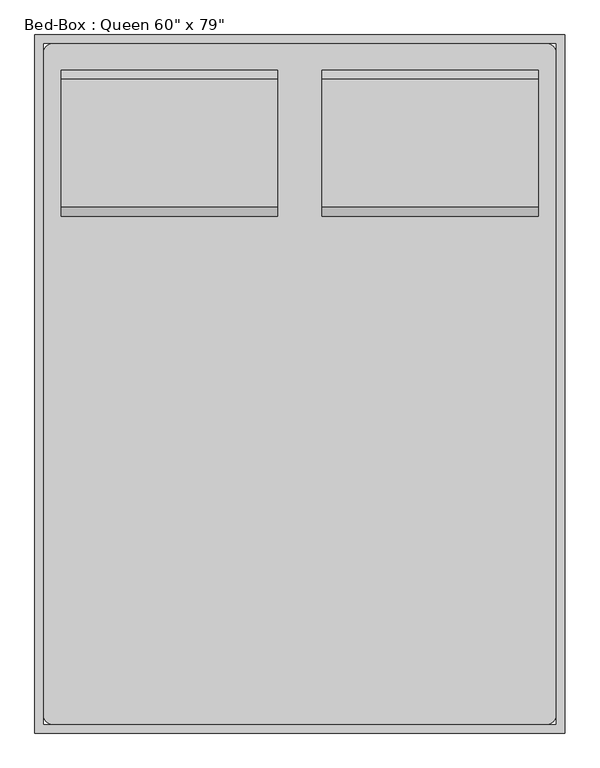
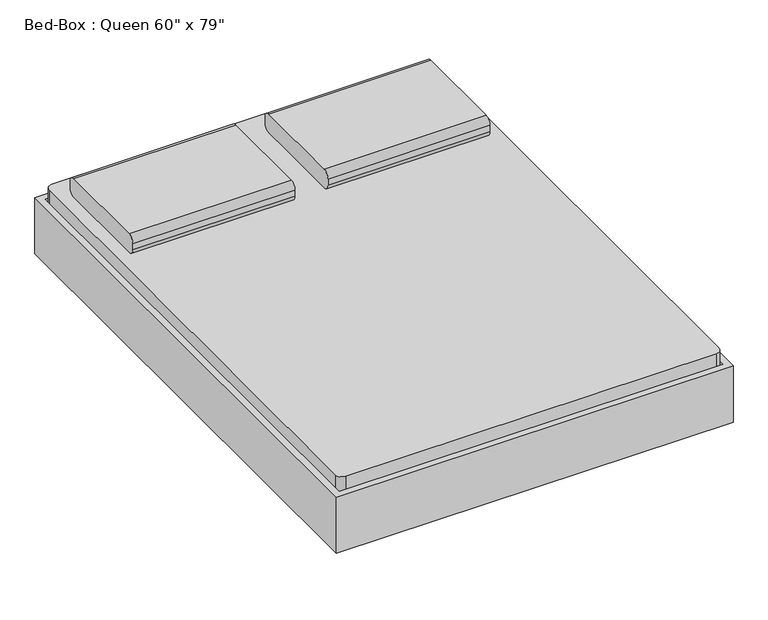
"""IFC4 building model written with IfcOpenShell, lengths in millimetres: furniture geometry."""

from ifc_helpers import new_model, si_unit, point, frame, frame_2d, origin, place, context, project, spatial, polyline, circle_curve, trimmed, segment, composite_curve, outline, extrude, source, transform, mapped, element, save
from ifc_brep_helpers import plane_surface, cylinder_surface, revolved_surface, advanced_brep


def furniture_1d2926bd(model_context):
    return source(origin(), model_context, "Body", "SolidModel", [
        extrude(outline(composite_curve([segment(polyline([(641.8704918, 406.4), (273.5704918, 406.4)]), True, "CONTINUOUS"), segment(trimmed(circle_curve(frame_2d((273.5704918, 431.8)), 25.4), [point((273.5704918, 406.4))], [point((248.1704918, 431.8))], False, "CARTESIAN"), True, "CONTINUOUS"), segment(polyline([(248.1704918, 431.8), (248.1704918, 457.2)]), True, "CONTINUOUS"), segment(trimmed(circle_curve(frame_2d((273.5704918, 457.2)), 25.4), [point((248.1704918, 457.2))], [point((273.5704918, 482.6))], False, "CARTESIAN"), True, "CONTINUOUS"), segment(polyline([(273.5704918, 482.6), (641.8704918, 482.6)]), True, "CONTINUOUS"), segment(trimmed(circle_curve(frame_2d((641.8704918, 457.2)), 25.4), [point((641.8704918, 482.6))], [point((667.2704918, 457.2))], False, "CARTESIAN"), True, "CONTINUOUS"), segment(polyline([(667.2704918, 457.2), (667.2704918, 431.8)]), True, "CONTINUOUS"), segment(trimmed(circle_curve(frame_2d((641.8704918, 431.8)), 25.4), [point((667.2704918, 431.8))], [point((641.8704918, 406.4))], False, "CARTESIAN"), True, "CONTINUOUS")], self_intersect=False)), frame((402.652459, 0.0, 0.0), z_axis=(1.0, 0.0, 0.0), x_axis=(0.0, 1.0, 0.0)), (0.0, 0.0, 1.0), 622.3),
        extrude(outline(composite_curve([segment(polyline([(641.8704918, 406.4), (273.5704918, 406.4)]), True, "CONTINUOUS"), segment(trimmed(circle_curve(frame_2d((273.5704918, 431.8)), 25.4), [point((273.5704918, 406.4))], [point((248.1704918, 431.8))], False, "CARTESIAN"), True, "CONTINUOUS"), segment(polyline([(248.1704918, 431.8), (248.1704918, 457.2)]), True, "CONTINUOUS"), segment(trimmed(circle_curve(frame_2d((273.5704918, 457.2)), 25.4), [point((248.1704918, 457.2))], [point((273.5704918, 482.6))], False, "CARTESIAN"), True, "CONTINUOUS"), segment(polyline([(273.5704918, 482.6), (641.8704918, 482.6)]), True, "CONTINUOUS"), segment(trimmed(circle_curve(frame_2d((641.8704918, 457.2)), 25.4), [point((641.8704918, 482.6))], [point((667.2704918, 457.2))], False, "CARTESIAN"), True, "CONTINUOUS"), segment(polyline([(667.2704918, 457.2), (667.2704918, 431.8)]), True, "CONTINUOUS"), segment(trimmed(circle_curve(frame_2d((641.8704918, 431.8)), 25.4), [point((667.2704918, 431.8))], [point((641.8704918, 406.4))], False, "CARTESIAN"), True, "CONTINUOUS")], self_intersect=False)), frame((-346.647541, 0.0, 0.0), z_axis=(1.0, 0.0, 0.0), x_axis=(0.0, 1.0, 0.0)), (0.0, 0.0, 1.0), 622.3),
        advanced_brep(
        [(-397.1231784, 514.8704918, 177.8), (-397.1231784, 438.6704918, 177.8), (-397.1231784, 438.6704918, 196.85), (-397.1231784, 514.8704918, 196.85), (-346.3231784, 514.8704918, 177.8), (-346.3231784, 438.6704918, 177.8), (-334.1869899, 438.6704918, 196.85), (-334.1869899, 514.8704918, 196.85), (-270.2523099, 514.8704918, 14.6654962), (-270.2523099, 438.6704918, 14.6654962), (-252.9871466, 438.6704918, 22.716374), (-252.9871466, 514.8704918, 22.716374), (-247.2320921, 438.6704918, 0.0), (-247.2320921, 514.8704918, 0.0), (-247.2320921, 438.6704918, 19.05), (-247.2320921, 514.8704918, 19.05), (-168.6195862, 514.8704918, 0.0), (-168.6195862, 438.6704918, 0.0), (-168.6195862, 438.6704918, 19.05), (-168.6195862, 514.8704918, 19.05), (-155.9195862, 438.6704918, 3.4029547), (-155.9195862, 514.8704918, 3.4029547), (-165.4445862, 438.6704918, 19.9007387), (-165.4445862, 514.8704918, 19.9007387), (-95.822541, 514.8704918, 38.1), (-95.822541, 438.6704918, 38.1), (-100.9269731, 438.6704918, 57.15), (-100.9269731, 514.8704918, 57.15), (774.4518216, 514.8704918, 38.1), (774.4518216, 438.6704918, 38.1), (779.5562537, 438.6704918, 57.15), (779.5562537, 514.8704918, 57.15), (834.5488669, 514.8704918, 3.4029547), (834.5488669, 438.6704918, 3.4029547), (844.0738669, 438.6704918, 19.9007387), (844.0738669, 514.8704918, 19.9007387), (847.2488669, 438.6704918, 0.0), (847.2488669, 514.8704918, 0.0), (847.2488669, 438.6704918, 19.05), (847.2488669, 514.8704918, 19.05), (925.8613728, 514.8704918, 0.0), (925.8613728, 438.6704918, 0.0), (925.8613728, 438.6704918, 19.05), (925.8613728, 514.8704918, 19.05), (948.8815906, 438.6704918, 14.6654962), (948.8815906, 514.8704918, 14.6654962), (931.6164272, 438.6704918, 22.716374), (931.6164272, 514.8704918, 22.716374), (1024.952459, 514.8704918, 177.8), (1024.952459, 438.6704918, 177.8), (1012.8162705, 438.6704918, 196.85), (1012.8162705, 514.8704918, 196.85), (1075.752459, 514.8704918, 177.8), (1075.752459, 514.8704918, 196.85), (1075.752459, 438.6704918, 196.85), (1075.752459, 438.6704918, 177.8)],
        [
            (0, 1),
            (1, 2),
            (2, 3),
            (3, 0),
            (0, 4),
            (4, 5),
            (5, 1),
            (5, 6),
            (6, 2),
            (6, 7),
            (7, 3),
            (7, 4),
            (4, 8),
            (8, 9),
            (9, 5),
            (9, 10),
            (10, 6),
            (10, 11),
            (11, 7),
            (11, 8),
            (12, 9, circle_curve(frame((-247.2320921, 438.6704918, 25.4), z_axis=(0.0, 1.0, 0.0), x_axis=(-0.9063077870366486, 0.0, -0.42261826174070233)), 25.4)),
            (8, 13, circle_curve(frame((-247.2320921, 514.8704918, 25.4), z_axis=(0.0, -1.0, 0.0), x_axis=(-0.9063077870366486, 0.0, -0.42261826174070233)), 25.4)),
            (13, 12),
            (14, 10, circle_curve(frame((-247.2320921, 438.6704918, 25.4), z_axis=(0.0, 1.0, 0.0), x_axis=(-0.9063077870366486, 0.0, -0.42261826174070233)), 6.35)),
            (12, 14),
            (15, 11, circle_curve(frame((-247.2320921, 514.8704918, 25.4), z_axis=(0.0, 1.0, 0.0), x_axis=(-0.9063077870366486, 0.0, -0.42261826174070233)), 6.35)),
            (14, 15),
            (15, 13),
            (13, 16),
            (16, 17),
            (17, 12),
            (17, 18),
            (18, 14),
            (18, 19),
            (19, 15),
            (19, 16),
            (20, 17, circle_curve(frame((-168.6195862, 438.6704918, 25.4), z_axis=(0.0, 1.0, 0.0), x_axis=(0.0, 0.0, -1.0)), 25.4)),
            (16, 21, circle_curve(frame((-168.6195862, 514.8704918, 25.4), z_axis=(0.0, -1.0, 0.0), x_axis=(0.0, 0.0, -1.0)), 25.4)),
            (21, 20),
            (22, 18, circle_curve(frame((-168.6195862, 438.6704918, 25.4), z_axis=(0.0, 1.0, 0.0), x_axis=(0.0, 0.0, -1.0)), 6.35)),
            (20, 22),
            (23, 19, circle_curve(frame((-168.6195862, 514.8704918, 25.4), z_axis=(0.0, 1.0, 0.0), x_axis=(0.0, 0.0, -1.0)), 6.35)),
            (22, 23),
            (23, 21),
            (21, 24),
            (24, 25),
            (25, 20),
            (25, 26),
            (26, 22),
            (26, 27),
            (27, 23),
            (27, 24),
            (24, 28),
            (28, 29),
            (29, 25),
            (29, 30),
            (30, 26),
            (30, 31),
            (31, 27),
            (31, 28),
            (28, 32),
            (32, 33),
            (33, 29),
            (33, 34),
            (34, 30),
            (34, 35),
            (35, 31),
            (35, 32),
            (36, 33, circle_curve(frame((847.2488669, 438.6704918, 25.4), z_axis=(0.0, 1.0, 0.0), x_axis=(-0.5000000000000463, 0.0, -0.8660254037844118)), 25.4)),
            (32, 37, circle_curve(frame((847.2488669, 514.8704918, 25.4), z_axis=(0.0, -1.0, 0.0), x_axis=(-0.5000000000000463, 0.0, -0.8660254037844118)), 25.4)),
            (37, 36),
            (38, 34, circle_curve(frame((847.2488669, 438.6704918, 25.4), z_axis=(0.0, 1.0, 0.0), x_axis=(-0.5000000000000463, 0.0, -0.8660254037844118)), 6.35)),
            (36, 38),
            (39, 35, circle_curve(frame((847.2488669, 514.8704918, 25.4), z_axis=(0.0, 1.0, 0.0), x_axis=(-0.5000000000000463, 0.0, -0.8660254037844118)), 6.35)),
            (38, 39),
            (39, 37),
            (37, 40),
            (40, 41),
            (41, 36),
            (41, 42),
            (42, 38),
            (42, 43),
            (43, 39),
            (43, 40),
            (44, 41, circle_curve(frame((925.8613728, 438.6704918, 25.4), z_axis=(0.0, 1.0, 0.0), x_axis=(0.0, 0.0, -1.0)), 25.4)),
            (40, 45, circle_curve(frame((925.8613728, 514.8704918, 25.4), z_axis=(0.0, -1.0, 0.0), x_axis=(0.0, 0.0, -1.0)), 25.4)),
            (45, 44),
            (46, 42, circle_curve(frame((925.8613728, 438.6704918, 25.4), z_axis=(0.0, 1.0, 0.0), x_axis=(0.0, 0.0, -1.0)), 6.35)),
            (44, 46),
            (47, 43, circle_curve(frame((925.8613728, 514.8704918, 25.4), z_axis=(0.0, 1.0, 0.0), x_axis=(0.0, 0.0, -1.0)), 6.35)),
            (46, 47),
            (47, 45),
            (45, 48),
            (48, 49),
            (49, 44),
            (49, 50),
            (50, 46),
            (50, 51),
            (51, 47),
            (51, 48),
            (52, 53),
            (53, 54),
            (54, 55),
            (55, 52),
            (48, 52),
            (55, 49),
            (54, 50),
            (53, 51),
        ],
        [
            plane_surface(frame((-397.1231784, 768.8704918, -152.9490627), z_axis=(-1.0, 0.0, 0.0), x_axis=(0.0, 1.0, 0.0))),
            plane_surface(frame((-397.1231784, 514.8704918, 177.8), z_axis=(0.0, 0.0, -1.0), x_axis=(1.0, 0.0, 0.0))),
            plane_surface(frame((-397.1231784, 438.6704918, 177.8), z_axis=(0.0, -1.0, 0.0), x_axis=(1.0, 0.0, 0.0))),
            plane_surface(frame((-397.1231784, 438.6704918, 196.85), z_axis=(0.0, 0.0, 1.0), x_axis=(1.0, 0.0, 0.0))),
            plane_surface(frame((-397.1231784, 514.8704918, 196.85), z_axis=(0.0, 1.0, 0.0), x_axis=(1.0, 0.0, 0.0))),
            plane_surface(frame((-346.3231784, 514.8704918, 177.8), z_axis=(-0.9063077870366485, 0.0, -0.4226182617407027), x_axis=(0.4226182617407027, 0.0, -0.9063077870366485))),
            plane_surface(frame((-346.3231784, 438.6704918, 177.8), z_axis=(0.0, -1.0, 0.0), x_axis=(0.4226182617407025, 0.0, -0.9063077870366486))),
            plane_surface(frame((-334.1869899, 438.6704918, 196.85), z_axis=(0.9063077870366484, 0.0, 0.4226182617407028), x_axis=(0.4226182617407028, 0.0, -0.9063077870366484))),
            plane_surface(frame((-334.1869899, 514.8704918, 196.85), z_axis=(0.0, 1.0, 0.0), x_axis=(0.42261826174070277, 0.0, -0.9063077870366485))),
            cylinder_surface(frame((-247.2320921, 768.8704918, 25.4), z_axis=(0.0, -1.0, 0.0), x_axis=(-0.9063077870366486, 0.0, -0.42261826174070233)), 25.4),
            plane_surface(frame((-247.2320921, 438.6704918, 25.4), z_axis=(0.0, -1.0, 0.0), x_axis=(-0.9063077870366486, 0.0, -0.42261826174070233))),
            revolved_surface(polyline([(-252.9871465476827, 438.6704918, 22.71637403794654), (-252.9871465476827, 514.8704918, 22.71637403794654)]), (-247.2320921, 768.8704918, 25.4), (0.0, -1.0, 0.0)),
            plane_surface(frame((-247.2320921, 514.8704918, 25.4), z_axis=(0.0, 1.0, 0.0), x_axis=(-0.9063077870366486, 0.0, -0.42261826174070233))),
            plane_surface(frame((-247.2320921, 514.8704918, 0.0), z_axis=(0.0, 0.0, -1.0), x_axis=(1.0, 0.0, 0.0))),
            plane_surface(frame((-247.2320921, 438.6704918, 0.0), z_axis=(0.0, -1.0, 0.0), x_axis=(1.0, 0.0, 0.0))),
            plane_surface(frame((-247.2320921, 438.6704918, 19.05), z_axis=(0.0, 0.0, 1.0), x_axis=(1.0, 0.0, 0.0))),
            plane_surface(frame((-247.2320921, 514.8704918, 19.05), z_axis=(0.0, 1.0, 0.0), x_axis=(1.0, 0.0, 0.0))),
            cylinder_surface(frame((-168.6195862, 768.8704918, 25.4), z_axis=(0.0, -1.0, 0.0), x_axis=(0.0, 0.0, -1.0)), 25.4),
            plane_surface(frame((-168.6195862, 438.6704918, 25.4), z_axis=(0.0, -1.0, 0.0), x_axis=(0.0, 0.0, -1.0))),
            revolved_surface(polyline([(-168.6195862, 438.6704918, 19.049999999999997), (-168.6195862, 514.8704918, 19.049999999999997)]), (-168.6195862, 768.8704918, 25.4), (0.0, -1.0, 0.0)),
            plane_surface(frame((-168.6195862, 514.8704918, 25.4), z_axis=(0.0, 1.0, 0.0), x_axis=(0.0, 0.0, -1.0))),
            plane_surface(frame((-155.9195862, 514.8704918, 3.4029547), z_axis=(0.49999999999988004, 0.0, -0.866025403784508), x_axis=(0.866025403784508, 0.0, 0.49999999999988004))),
            plane_surface(frame((-155.9195862, 438.6704918, 3.4029547), z_axis=(0.0, -1.0, 0.0), x_axis=(0.8660254037845078, 0.0, 0.49999999999988026))),
            plane_surface(frame((-165.4445862, 438.6704918, 19.9007387), z_axis=(-0.4999999999998799, 0.0, 0.866025403784508), x_axis=(0.866025403784508, 0.0, 0.4999999999998799))),
            plane_surface(frame((-165.4445862, 514.8704918, 19.9007387), z_axis=(0.0, 1.0, 0.0), x_axis=(0.8660254037845075, 0.0, 0.49999999999988076))),
            plane_surface(frame((-95.822541, 514.8704918, 38.1), z_axis=(0.0, 0.0, -1.0), x_axis=(1.0, 0.0, 0.0))),
            plane_surface(frame((-95.822541, 438.6704918, 38.1), z_axis=(0.0, -1.0, 0.0), x_axis=(1.0, 0.0, 0.0))),
            plane_surface(frame((-100.9269731, 438.6704918, 57.15), z_axis=(0.0, 0.0, 1.0), x_axis=(1.0, 0.0, 0.0))),
            plane_surface(frame((-100.9269731, 514.8704918, 57.15), z_axis=(0.0, 1.0, 0.0), x_axis=(1.0, 0.0, 0.0))),
            plane_surface(frame((774.4518216, 514.8704918, 38.1), z_axis=(-0.5000000000000455, 0.0, -0.8660254037844125), x_axis=(0.8660254037844125, 0.0, -0.5000000000000455))),
            plane_surface(frame((774.4518216, 438.6704918, 38.1), z_axis=(0.0, -1.0, 0.0), x_axis=(0.866025403784412, 0.0, -0.5000000000000463))),
            plane_surface(frame((779.5562537, 438.6704918, 57.15), z_axis=(0.5000000000000466, 0.0, 0.8660254037844117), x_axis=(0.8660254037844117, 0.0, -0.5000000000000466))),
            plane_surface(frame((779.5562537, 514.8704918, 57.15), z_axis=(0.0, 1.0, 0.0), x_axis=(0.8660254037844115, 0.0, -0.5000000000000471))),
            cylinder_surface(frame((847.2488669, 768.8704918, 25.4), z_axis=(0.0, -1.0, 0.0), x_axis=(-0.5000000000000463, 0.0, -0.8660254037844118)), 25.4),
            plane_surface(frame((847.2488669, 438.6704918, 25.4), z_axis=(0.0, -1.0000000000000002, 0.0), x_axis=(-0.5000000000000464, 0.0, -0.866025403784412))),
            revolved_surface(polyline([(844.0738668999998, 438.6704918, 19.90073868596898), (844.0738668999998, 514.8704918, 19.90073868596898)]), (847.2488669, 768.8704918, 25.4), (0.0, -1.0, 0.0)),
            plane_surface(frame((847.2488669, 514.8704918, 25.4), z_axis=(0.0, 1.0000000000000002, 0.0), x_axis=(-0.5000000000000464, 0.0, -0.866025403784412))),
            plane_surface(frame((847.2488669, 514.8704918, 0.0), z_axis=(0.0, 0.0, -1.0), x_axis=(1.0, 0.0, 0.0))),
            plane_surface(frame((847.2488669, 438.6704918, 0.0), z_axis=(0.0, -1.0, 0.0), x_axis=(1.0, 0.0, 0.0))),
            plane_surface(frame((847.2488669, 438.6704918, 19.05), z_axis=(0.0, 0.0, 1.0), x_axis=(1.0, 0.0, 0.0))),
            plane_surface(frame((847.2488669, 514.8704918, 19.05), z_axis=(0.0, 1.0, 0.0), x_axis=(1.0, 0.0, 0.0))),
            cylinder_surface(frame((925.8613728, 768.8704918, 25.4), z_axis=(0.0, -1.0, 0.0), x_axis=(0.0, 0.0, -1.0)), 25.4),
            plane_surface(frame((925.8613728, 438.6704918, 25.4), z_axis=(0.0, -1.0, 0.0), x_axis=(0.0, 0.0, -1.0))),
            revolved_surface(polyline([(925.8613728, 438.6704918, 19.049999999999997), (925.8613728, 514.8704918, 19.049999999999997)]), (925.8613728, 768.8704918, 25.4), (0.0, -1.0, 0.0)),
            plane_surface(frame((925.8613728, 514.8704918, 25.4), z_axis=(0.0, 1.0, 0.0), x_axis=(0.0, 0.0, -1.0))),
            plane_surface(frame((948.8815906, 514.8704918, 14.6654962), z_axis=(0.90630778703668, 0.0, -0.42261826174063505), x_axis=(0.42261826174063505, 0.0, 0.90630778703668))),
            plane_surface(frame((948.8815906, 438.6704918, 14.6654962), z_axis=(0.0, -1.0, 0.0), x_axis=(0.42261826174063566, 0.0, 0.9063077870366797))),
            plane_surface(frame((931.6164272, 438.6704918, 22.716374), z_axis=(-0.9063077870366801, 0.0, 0.42261826174063477), x_axis=(0.42261826174063477, 0.0, 0.9063077870366801))),
            plane_surface(frame((931.6164272, 514.8704918, 22.716374), z_axis=(0.0, 1.0, 0.0), x_axis=(0.4226182617406345, 0.0, 0.9063077870366802))),
            plane_surface(frame((1075.752459, 768.8704918, -152.9490627), z_axis=(1.0, 0.0, 0.0), x_axis=(0.0, 1.0, 0.0))),
            plane_surface(frame((1024.952459, 514.8704918, 177.8), z_axis=(0.0, 0.0, -1.0), x_axis=(1.0, 0.0, 0.0))),
            plane_surface(frame((1024.952459, 438.6704918, 177.8), z_axis=(0.0, -1.0, 0.0), x_axis=(1.0, 0.0, 0.0))),
            plane_surface(frame((1012.8162705, 438.6704918, 196.85), z_axis=(0.0, 0.0, 1.0), x_axis=(1.0, 0.0, 0.0))),
            plane_surface(frame((1012.8162705, 514.8704918, 196.85), z_axis=(0.0, 1.0, 0.0), x_axis=(1.0, 0.0, 0.0))),
        ],
        [
            (0, [[1, 2, 3, 4]]),
            (1, [[-1, 5, 6, 7]]),
            (2, [[-2, -7, 8, 9]]),
            (3, [[-3, -9, 10, 11]]),
            (4, [[-4, -11, 12, -5]]),
            (5, [[-6, 13, 14, 15]]),
            (6, [[-8, -15, 16, 17]]),
            (7, [[-10, -17, 18, 19]]),
            (8, [[-12, -19, 20, -13]]),
            (9, [[21, -14, 22, 23]]),
            (10, [[24, -16, -21, 25]]),
            (11, [[26, -18, -24, 27]]),
            (12, [[-22, -20, -26, 28]]),
            (13, [[-23, 29, 30, 31]]),
            (14, [[-25, -31, 32, 33]]),
            (15, [[-27, -33, 34, 35]]),
            (16, [[-28, -35, 36, -29]]),
            (17, [[37, -30, 38, 39]]),
            (18, [[40, -32, -37, 41]]),
            (19, [[42, -34, -40, 43]]),
            (20, [[-38, -36, -42, 44]]),
            (21, [[-39, 45, 46, 47]]),
            (22, [[-41, -47, 48, 49]]),
            (23, [[-43, -49, 50, 51]]),
            (24, [[-44, -51, 52, -45]]),
            (25, [[-46, 53, 54, 55]]),
            (26, [[-48, -55, 56, 57]]),
            (27, [[-50, -57, 58, 59]]),
            (28, [[-52, -59, 60, -53]]),
            (29, [[-54, 61, 62, 63]]),
            (30, [[-56, -63, 64, 65]]),
            (31, [[-58, -65, 66, 67]]),
            (32, [[-60, -67, 68, -61]]),
            (33, [[69, -62, 70, 71]]),
            (34, [[72, -64, -69, 73]]),
            (35, [[74, -66, -72, 75]]),
            (36, [[-70, -68, -74, 76]]),
            (37, [[-71, 77, 78, 79]]),
            (38, [[-73, -79, 80, 81]]),
            (39, [[-75, -81, 82, 83]]),
            (40, [[-76, -83, 84, -77]]),
            (41, [[85, -78, 86, 87]]),
            (42, [[88, -80, -85, 89]]),
            (43, [[90, -82, -88, 91]]),
            (44, [[-86, -84, -90, 92]]),
            (45, [[-87, 93, 94, 95]]),
            (46, [[-89, -95, 96, 97]]),
            (47, [[-91, -97, 98, 99]]),
            (48, [[-92, -99, 100, -93]]),
            (49, [[101, 102, 103, 104]]),
            (50, [[-94, 105, -104, 106]]),
            (51, [[-96, -106, -103, 107]]),
            (52, [[-98, -107, -102, 108]]),
            (53, [[-100, -108, -101, -105]]),
        ],
    ),
        extrude(outline(composite_curve([segment(polyline([(-372.047541, 743.4704918), (1050.352459, 743.4704918)]), True, "CONTINUOUS"), segment(trimmed(circle_curve(frame_2d((1050.352459, 718.0704918)), 25.4), [point((1050.352459, 743.4704918))], [point((1075.752459, 718.0704918))], False, "CARTESIAN"), True, "CONTINUOUS"), segment(polyline([(1075.752459, 718.0704918), (1075.752459, -1186.9295082)]), True, "CONTINUOUS"), segment(trimmed(circle_curve(frame_2d((1050.352459, -1186.9295082)), 25.4), [point((1075.752459, -1186.9295082))], [point((1050.352459, -1212.3295082))], False, "CARTESIAN"), True, "CONTINUOUS"), segment(polyline([(1050.352459, -1212.3295082), (-372.047541, -1212.3295082)]), True, "CONTINUOUS"), segment(trimmed(circle_curve(frame_2d((-372.047541, -1186.9295082)), 25.4), [point((-372.047541, -1212.3295082))], [point((-397.447541, -1186.9295082))], False, "CARTESIAN"), True, "CONTINUOUS"), segment(polyline([(-397.447541, -1186.9295082), (-397.447541, 718.0704918)]), True, "CONTINUOUS"), segment(trimmed(circle_curve(frame_2d((-372.047541, 718.0704918)), 25.4), [point((-397.447541, 718.0704918))], [point((-372.047541, 743.4704918))], False, "CARTESIAN"), True, "CONTINUOUS")], self_intersect=False)), frame((0.0, 0.0, 203.2), z_axis=(0.0, 0.0, 1.0), x_axis=(1.0, 0.0, 0.0)), (0.0, 0.0, 1.0), 203.2),
        advanced_brep(
        [(-397.447541, -932.9295082, 196.85), (-397.447541, -932.9295082, 177.8), (-397.447541, -1009.1295082, 177.8), (-397.447541, -1009.1295082, 196.85), (-334.5113525, -932.9295082, 196.85), (-346.647541, -932.9295082, 177.8), (-346.647541, -1009.1295082, 177.8), (-334.5113525, -1009.1295082, 196.85), (-253.3115092, -932.9295082, 22.716374), (-270.5766725, -932.9295082, 14.6654962), (-270.5766725, -1009.1295082, 14.6654962), (-253.3115092, -1009.1295082, 22.716374), (-247.5564547, -932.9295082, 0.0), (-247.5564547, -932.9295082, 19.05), (-247.5564547, -1009.1295082, 0.0), (-247.5564547, -1009.1295082, 19.05), (-168.9439489, -932.9295082, 19.05), (-168.9439489, -932.9295082, 0.0), (-168.9439489, -1009.1295082, 0.0), (-168.9439489, -1009.1295082, 19.05), (-156.2439489, -932.9295082, 3.4029547), (-165.7689489, -932.9295082, 19.9007387), (-156.2439489, -1009.1295082, 3.4029547), (-165.7689489, -1009.1295082, 19.9007387), (-101.2513357, -932.9295082, 57.15), (-96.1469036, -932.9295082, 38.1), (-96.1469036, -1009.1295082, 38.1), (-101.2513357, -1009.1295082, 57.15), (779.5562537, -932.9295082, 57.15), (774.4518216, -932.9295082, 38.1), (774.4518216, -1009.1295082, 38.1), (779.5562537, -1009.1295082, 57.15), (844.0738669, -932.9295082, 19.9007387), (834.5488669, -932.9295082, 3.4029547), (834.5488669, -1009.1295082, 3.4029547), (844.0738669, -1009.1295082, 19.9007387), (847.2488669, -932.9295082, 0.0), (847.2488669, -932.9295082, 19.05), (847.2488669, -1009.1295082, 0.0), (847.2488669, -1009.1295082, 19.05), (925.8613728, -932.9295082, 19.05), (925.8613728, -932.9295082, 0.0), (925.8613728, -1009.1295082, 0.0), (925.8613728, -1009.1295082, 19.05), (948.8815906, -932.9295082, 14.6654962), (931.6164272, -932.9295082, 22.716374), (948.8815906, -1009.1295082, 14.6654962), (931.6164272, -1009.1295082, 22.716374), (1012.8162705, -932.9295082, 196.85), (1024.952459, -932.9295082, 177.8), (1024.952459, -1009.1295082, 177.8), (1012.8162705, -1009.1295082, 196.85), (1075.752459, -932.9295082, 196.85), (1075.752459, -1009.1295082, 196.85), (1075.752459, -1009.1295082, 177.8), (1075.752459, -932.9295082, 177.8)],
        [
            (0, 1),
            (1, 2),
            (2, 3),
            (3, 0),
            (0, 4),
            (4, 5),
            (5, 1),
            (5, 6),
            (6, 2),
            (6, 7),
            (7, 3),
            (7, 4),
            (4, 8),
            (8, 9),
            (9, 5),
            (9, 10),
            (10, 6),
            (10, 11),
            (11, 7),
            (11, 8),
            (12, 9, circle_curve(frame((-247.5564547, -932.9295082, 25.4), z_axis=(0.0, 1.0, 0.0), x_axis=(-0.906307787036663, 0.0, -0.4226182617406713)), 25.4)),
            (8, 13, circle_curve(frame((-247.5564547, -932.9295082, 25.4), z_axis=(0.0, -1.0, 0.0), x_axis=(-0.906307787036663, 0.0, -0.4226182617406713)), 6.35)),
            (13, 12),
            (14, 10, circle_curve(frame((-247.5564547, -1009.1295082, 25.4), z_axis=(0.0, 1.0, 0.0), x_axis=(-0.906307787036663, 0.0, -0.4226182617406713)), 25.4)),
            (12, 14),
            (15, 11, circle_curve(frame((-247.5564547, -1009.1295082, 25.4), z_axis=(0.0, 1.0, 0.0), x_axis=(-0.906307787036663, 0.0, -0.4226182617406713)), 6.35)),
            (14, 15),
            (15, 13),
            (13, 16),
            (16, 17),
            (17, 12),
            (17, 18),
            (18, 14),
            (18, 19),
            (19, 15),
            (19, 16),
            (20, 17, circle_curve(frame((-168.9439489, -932.9295082, 25.4), z_axis=(0.0, 1.0, 0.0), x_axis=(0.0, 0.0, -1.0)), 25.4)),
            (16, 21, circle_curve(frame((-168.9439489, -932.9295082, 25.4), z_axis=(0.0, -1.0, 0.0), x_axis=(0.0, 0.0, -1.0)), 6.35)),
            (21, 20),
            (22, 18, circle_curve(frame((-168.9439489, -1009.1295082, 25.4), z_axis=(0.0, 1.0, 0.0), x_axis=(0.0, 0.0, -1.0)), 25.4)),
            (20, 22),
            (23, 19, circle_curve(frame((-168.9439489, -1009.1295082, 25.4), z_axis=(0.0, 1.0, 0.0), x_axis=(0.0, 0.0, -1.0)), 6.35)),
            (22, 23),
            (23, 21),
            (21, 24),
            (24, 25),
            (25, 20),
            (25, 26),
            (26, 22),
            (26, 27),
            (27, 23),
            (27, 24),
            (24, 28),
            (28, 29),
            (29, 25),
            (29, 30),
            (30, 26),
            (30, 31),
            (31, 27),
            (31, 28),
            (28, 32),
            (32, 33),
            (33, 29),
            (33, 34),
            (34, 30),
            (34, 35),
            (35, 31),
            (35, 32),
            (36, 33, circle_curve(frame((847.2488669, -932.9295082, 25.4), z_axis=(0.0, 1.0, 0.0), x_axis=(-0.5000000000000479, 0.0, -0.866025403784411)), 25.4)),
            (32, 37, circle_curve(frame((847.2488669, -932.9295082, 25.4), z_axis=(0.0, -1.0, 0.0), x_axis=(-0.5000000000000479, 0.0, -0.866025403784411)), 6.35)),
            (37, 36),
            (38, 34, circle_curve(frame((847.2488669, -1009.1295082, 25.4), z_axis=(0.0, 1.0, 0.0), x_axis=(-0.5000000000000479, 0.0, -0.866025403784411)), 25.4)),
            (36, 38),
            (39, 35, circle_curve(frame((847.2488669, -1009.1295082, 25.4), z_axis=(0.0, 1.0, 0.0), x_axis=(-0.5000000000000479, 0.0, -0.866025403784411)), 6.35)),
            (38, 39),
            (39, 37),
            (37, 40),
            (40, 41),
            (41, 36),
            (41, 42),
            (42, 38),
            (42, 43),
            (43, 39),
            (43, 40),
            (44, 41, circle_curve(frame((925.8613728, -932.9295082, 25.4), z_axis=(0.0, 1.0, 0.0), x_axis=(0.0, 0.0, -1.0)), 25.4)),
            (40, 45, circle_curve(frame((925.8613728, -932.9295082, 25.4), z_axis=(0.0, -1.0, 0.0), x_axis=(0.0, 0.0, -1.0)), 6.35)),
            (45, 44),
            (46, 42, circle_curve(frame((925.8613728, -1009.1295082, 25.4), z_axis=(0.0, 1.0, 0.0), x_axis=(0.0, 0.0, -1.0)), 25.4)),
            (44, 46),
            (47, 43, circle_curve(frame((925.8613728, -1009.1295082, 25.4), z_axis=(0.0, 1.0, 0.0), x_axis=(0.0, 0.0, -1.0)), 6.35)),
            (46, 47),
            (47, 45),
            (45, 48),
            (48, 49),
            (49, 44),
            (49, 50),
            (50, 46),
            (50, 51),
            (51, 47),
            (51, 48),
            (52, 53),
            (53, 54),
            (54, 55),
            (55, 52),
            (48, 52),
            (55, 49),
            (54, 50),
            (53, 51),
        ],
        [
            plane_surface(frame((-397.447541, -1237.7295082, -127.5947323), z_axis=(-1.0, 0.0, 0.0), x_axis=(0.0, 1.0, 0.0))),
            plane_surface(frame((-397.447541, -932.9295082, 196.85), z_axis=(0.0, 1.0, 0.0), x_axis=(1.0, 0.0, 0.0))),
            plane_surface(frame((-397.447541, -932.9295082, 177.8), z_axis=(0.0, 0.0, -1.0), x_axis=(1.0, 0.0, 0.0))),
            plane_surface(frame((-397.447541, -1009.1295082, 177.8), z_axis=(0.0, -1.0, 0.0), x_axis=(1.0, 0.0, 0.0))),
            plane_surface(frame((-397.447541, -1009.1295082, 196.85), z_axis=(0.0, 0.0, 1.0), x_axis=(1.0, 0.0, 0.0))),
            plane_surface(frame((-334.5113525, -932.9295082, 196.85), z_axis=(0.0, 1.0, 0.0), x_axis=(0.4226182617406707, 0.0, -0.9063077870366634))),
            plane_surface(frame((-346.647541, -932.9295082, 177.8), z_axis=(-0.9063077870366635, 0.0, -0.4226182617406707), x_axis=(0.4226182617406707, 0.0, -0.9063077870366635))),
            plane_surface(frame((-346.647541, -1009.1295082, 177.8), z_axis=(0.0, -1.0, 0.0), x_axis=(0.422618261740671, 0.0, -0.9063077870366633))),
            plane_surface(frame((-334.5113525, -1009.1295082, 196.85), z_axis=(0.9063077870366633, 0.0, 0.42261826174067113), x_axis=(0.42261826174067113, 0.0, -0.9063077870366633))),
            plane_surface(frame((-247.5564547, -932.9295082, 25.4), z_axis=(0.0, 1.0, 0.0), x_axis=(-0.906307787036663, 0.0, -0.4226182617406713))),
            cylinder_surface(frame((-247.5564547, -1237.7295082, 25.4), z_axis=(0.0, -1.0, 0.0), x_axis=(-0.906307787036663, 0.0, -0.4226182617406713)), 25.4),
            plane_surface(frame((-247.5564547, -1009.1295082, 25.4), z_axis=(0.0, -1.0, 0.0), x_axis=(-0.906307787036663, 0.0, -0.4226182617406713))),
            revolved_surface(polyline([(-253.3115091476828, -1009.1295082, 22.716374037946736), (-253.3115091476828, -932.9295082, 22.716374037946736)]), (-247.5564547, -1237.7295082, 25.4), (0.0, -1.0, 0.0)),
            plane_surface(frame((-247.5564547, -932.9295082, 19.05), z_axis=(0.0, 1.0, 0.0), x_axis=(1.0, 0.0, 0.0))),
            plane_surface(frame((-247.5564547, -932.9295082, 0.0), z_axis=(0.0, 0.0, -1.0), x_axis=(1.0, 0.0, 0.0))),
            plane_surface(frame((-247.5564547, -1009.1295082, 0.0), z_axis=(0.0, -1.0, 0.0), x_axis=(1.0, 0.0, 0.0))),
            plane_surface(frame((-247.5564547, -1009.1295082, 19.05), z_axis=(0.0, 0.0, 1.0), x_axis=(1.0, 0.0, 0.0))),
            plane_surface(frame((-168.9439489, -932.9295082, 25.4), z_axis=(0.0, 1.0, 0.0), x_axis=(0.0, 0.0, -1.0))),
            cylinder_surface(frame((-168.9439489, -1237.7295082, 25.4), z_axis=(0.0, -1.0, 0.0), x_axis=(0.0, 0.0, -1.0)), 25.4),
            plane_surface(frame((-168.9439489, -1009.1295082, 25.4), z_axis=(0.0, -1.0, 0.0), x_axis=(0.0, 0.0, -1.0))),
            revolved_surface(polyline([(-168.9439489, -1009.1295082, 19.049999999999997), (-168.9439489, -932.9295082, 19.049999999999997)]), (-168.9439489, -1237.7295082, 25.4), (0.0, -1.0, 0.0)),
            plane_surface(frame((-165.7689489, -932.9295082, 19.9007387), z_axis=(0.0, 1.0, 0.0), x_axis=(0.8660254037844788, 0.0, 0.4999999999999306))),
            plane_surface(frame((-156.2439489, -932.9295082, 3.4029547), z_axis=(0.49999999999993017, 0.0, -0.866025403784479), x_axis=(0.866025403784479, 0.0, 0.49999999999993017))),
            plane_surface(frame((-156.2439489, -1009.1295082, 3.4029547), z_axis=(0.0, -1.0, 0.0), x_axis=(0.8660254037844785, 0.0, 0.49999999999993106))),
            plane_surface(frame((-165.7689489, -1009.1295082, 19.9007387), z_axis=(-0.4999999999999309, 0.0, 0.8660254037844786), x_axis=(0.8660254037844786, 0.0, 0.4999999999999309))),
            plane_surface(frame((-101.2513357, -932.9295082, 57.15), z_axis=(0.0, 1.0, 0.0), x_axis=(1.0, 0.0, 0.0))),
            plane_surface(frame((-96.1469036, -932.9295082, 38.1), z_axis=(0.0, 0.0, -1.0), x_axis=(1.0, 0.0, 0.0))),
            plane_surface(frame((-96.1469036, -1009.1295082, 38.1), z_axis=(0.0, -1.0, 0.0), x_axis=(1.0, 0.0, 0.0))),
            plane_surface(frame((-101.2513357, -1009.1295082, 57.15), z_axis=(0.0, 0.0, 1.0), x_axis=(1.0, 0.0, 0.0))),
            plane_surface(frame((779.5562537, -932.9295082, 57.15), z_axis=(0.0, 1.0000000000000002, 0.0), x_axis=(0.8660254037844106, 0.0, -0.5000000000000487))),
            plane_surface(frame((774.4518216, -932.9295082, 38.1), z_axis=(-0.5000000000000477, 0.0, -0.8660254037844112), x_axis=(0.8660254037844112, 0.0, -0.5000000000000477))),
            plane_surface(frame((774.4518216, -1009.1295082, 38.1), z_axis=(0.0, -1.0000000000000002, 0.0), x_axis=(0.8660254037844105, 0.0, -0.500000000000049))),
            plane_surface(frame((779.5562537, -1009.1295082, 57.15), z_axis=(0.5000000000000498, 0.0, 0.8660254037844098), x_axis=(0.8660254037844098, 0.0, -0.5000000000000498))),
            plane_surface(frame((847.2488669, -932.9295082, 25.4), z_axis=(0.0, 1.0000000000000002, 0.0), x_axis=(-0.500000000000048, 0.0, -0.8660254037844111))),
            cylinder_surface(frame((847.2488669, -1237.7295082, 25.4), z_axis=(0.0, -1.0, 0.0), x_axis=(-0.5000000000000479, 0.0, -0.866025403784411)), 25.4),
            plane_surface(frame((847.2488669, -1009.1295082, 25.4), z_axis=(0.0, -1.0000000000000002, 0.0), x_axis=(-0.500000000000048, 0.0, -0.8660254037844111))),
            revolved_surface(polyline([(844.0738668999998, -1009.1295082, 19.90073868596899), (844.0738668999998, -932.9295082, 19.90073868596899)]), (847.2488669, -1237.7295082, 25.4), (0.0, -1.0, 0.0)),
            plane_surface(frame((847.2488669, -932.9295082, 19.05), z_axis=(0.0, 1.0, 0.0), x_axis=(1.0, 0.0, 0.0))),
            plane_surface(frame((847.2488669, -932.9295082, 0.0), z_axis=(0.0, 0.0, -1.0), x_axis=(1.0, 0.0, 0.0))),
            plane_surface(frame((847.2488669, -1009.1295082, 0.0), z_axis=(0.0, -1.0, 0.0), x_axis=(1.0, 0.0, 0.0))),
            plane_surface(frame((847.2488669, -1009.1295082, 19.05), z_axis=(0.0, 0.0, 1.0), x_axis=(1.0, 0.0, 0.0))),
            plane_surface(frame((925.8613728, -932.9295082, 25.4), z_axis=(0.0, 1.0, 0.0), x_axis=(0.0, 0.0, -1.0))),
            cylinder_surface(frame((925.8613728, -1237.7295082, 25.4), z_axis=(0.0, -1.0, 0.0), x_axis=(0.0, 0.0, -1.0)), 25.4),
            plane_surface(frame((925.8613728, -1009.1295082, 25.4), z_axis=(0.0, -1.0, 0.0), x_axis=(0.0, 0.0, -1.0))),
            revolved_surface(polyline([(925.8613728, -1009.1295082, 19.049999999999997), (925.8613728, -932.9295082, 19.049999999999997)]), (925.8613728, -1237.7295082, 25.4), (0.0, -1.0, 0.0)),
            plane_surface(frame((931.6164272, -932.9295082, 22.716374), z_axis=(0.0, 1.0, 0.0), x_axis=(0.4226182617405411, 0.0, 0.9063077870367238))),
            plane_surface(frame((948.8815906, -932.9295082, 14.6654962), z_axis=(0.9063077870367237, 0.0, -0.4226182617405414), x_axis=(0.4226182617405414, 0.0, 0.9063077870367237))),
            plane_surface(frame((948.8815906, -1009.1295082, 14.6654962), z_axis=(0.0, -1.0, 0.0), x_axis=(0.42261826174054123, 0.0, 0.9063077870367238))),
            plane_surface(frame((931.6164272, -1009.1295082, 22.716374), z_axis=(-0.9063077870367237, 0.0, 0.4226182617405414), x_axis=(0.4226182617405414, 0.0, 0.9063077870367237))),
            plane_surface(frame((1075.752459, -1237.7295082, -127.5947323), z_axis=(1.0, 0.0, 0.0), x_axis=(0.0, 1.0, 0.0))),
            plane_surface(frame((1012.8162705, -932.9295082, 196.85), z_axis=(0.0, 1.0, 0.0), x_axis=(1.0, 0.0, 0.0))),
            plane_surface(frame((1024.952459, -932.9295082, 177.8), z_axis=(0.0, 0.0, -1.0), x_axis=(1.0, 0.0, 0.0))),
            plane_surface(frame((1024.952459, -1009.1295082, 177.8), z_axis=(0.0, -1.0, 0.0), x_axis=(1.0, 0.0, 0.0))),
            plane_surface(frame((1012.8162705, -1009.1295082, 196.85), z_axis=(0.0, 0.0, 1.0), x_axis=(1.0, 0.0, 0.0))),
        ],
        [
            (0, [[1, 2, 3, 4]]),
            (1, [[-1, 5, 6, 7]]),
            (2, [[-2, -7, 8, 9]]),
            (3, [[-3, -9, 10, 11]]),
            (4, [[-4, -11, 12, -5]]),
            (5, [[-6, 13, 14, 15]]),
            (6, [[-8, -15, 16, 17]]),
            (7, [[-10, -17, 18, 19]]),
            (8, [[-12, -19, 20, -13]]),
            (9, [[21, -14, 22, 23]]),
            (10, [[24, -16, -21, 25]]),
            (11, [[26, -18, -24, 27]]),
            (12, [[-22, -20, -26, 28]]),
            (13, [[-23, 29, 30, 31]]),
            (14, [[-25, -31, 32, 33]]),
            (15, [[-27, -33, 34, 35]]),
            (16, [[-28, -35, 36, -29]]),
            (17, [[37, -30, 38, 39]]),
            (18, [[40, -32, -37, 41]]),
            (19, [[42, -34, -40, 43]]),
            (20, [[-38, -36, -42, 44]]),
            (21, [[-39, 45, 46, 47]]),
            (22, [[-41, -47, 48, 49]]),
            (23, [[-43, -49, 50, 51]]),
            (24, [[-44, -51, 52, -45]]),
            (25, [[-46, 53, 54, 55]]),
            (26, [[-48, -55, 56, 57]]),
            (27, [[-50, -57, 58, 59]]),
            (28, [[-52, -59, 60, -53]]),
            (29, [[-54, 61, 62, 63]]),
            (30, [[-56, -63, 64, 65]]),
            (31, [[-58, -65, 66, 67]]),
            (32, [[-60, -67, 68, -61]]),
            (33, [[69, -62, 70, 71]]),
            (34, [[72, -64, -69, 73]]),
            (35, [[74, -66, -72, 75]]),
            (36, [[-70, -68, -74, 76]]),
            (37, [[-71, 77, 78, 79]]),
            (38, [[-73, -79, 80, 81]]),
            (39, [[-75, -81, 82, 83]]),
            (40, [[-76, -83, 84, -77]]),
            (41, [[85, -78, 86, 87]]),
            (42, [[88, -80, -85, 89]]),
            (43, [[90, -82, -88, 91]]),
            (44, [[-86, -84, -90, 92]]),
            (45, [[-87, 93, 94, 95]]),
            (46, [[-89, -95, 96, 97]]),
            (47, [[-91, -97, 98, 99]]),
            (48, [[-92, -99, 100, -93]]),
            (49, [[101, 102, 103, 104]]),
            (50, [[-94, 105, -104, 106]]),
            (51, [[-96, -106, -103, 107]]),
            (52, [[-98, -107, -102, 108]]),
            (53, [[-100, -108, -101, -105]]),
        ],
    ),
        extrude(outline(polyline([(1101.152459, 768.8704918), (1101.152459, -1237.7295082), (-422.847541, -1237.7295082), (-422.847541, 768.8704918), (1101.152459, 768.8704918)]), holes=[polyline([(1075.752459, 743.4704918), (-397.447541, 743.4704918), (-397.447541, -1212.3295082), (1075.752459, -1212.3295082), (1075.752459, 743.4704918)])]), frame((0.0, 0.0, 127.0), z_axis=(0.0, 0.0, 1.0), x_axis=(1.0, 0.0, 0.0)), (0.0, 0.0, 1.0), 228.6),
    ])


if __name__ == "__main__":
    model = new_model("IFC4")
    model_context = context("Model", 3, world=origin())
    ifc_project = project(units=[si_unit("LENGTHUNIT", "METRE", prefix="MILLI")], contexts=[model_context])
    site = spatial("IfcSite", under=ifc_project)
    building = spatial("IfcBuilding", under=site)
    placement = place(None, origin())
    furniture_shape = furniture_1d2926bd(model_context)
    element("IfcFurniture", 1, ObjectType="Bed-Box : Queen 60\" x 79\"", at=placement, inside=building, context=model_context, shape_type="MappedRepresentation", body=[
        mapped(furniture_shape, transform((0.0, 0.0, 0.0), x_axis=(1.0, 0.0, 0.0), y_axis=(0.0, 1.0, 0.0), z_axis=(0.0, 0.0, 1.0))),
    ])
    save(model, "model.ifc")

# Revit data of these elements
# Type "Bed-Box : Queen 60\" x 79\""
#   Assembly Code = "E2020200"
#   Length = 6' - 7"
#   Width = 5' - 0"
#   Frame Material = Birch
#   Mattress Material = Sash
#   Default Elevation = 0
# Element 1 (IfcFurniture, "Bed-Box : Queen 60\" x 79\"")
#   Materials on its faces: "Birch", "Sash"
# Materials
#   "Birch": class "Wood", colour RGB 224 178 126, transparency 0, Description = "Betula Alleghaniensis", Cost = 0
#   "Sash": class "Wood", colour RGB 224 178 126, transparency 0
